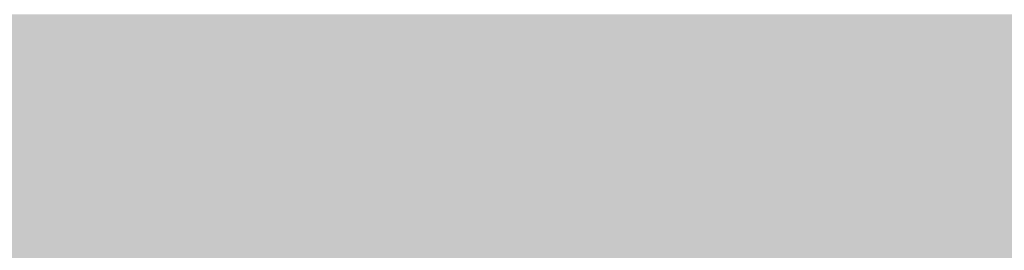
# Model space of a CAD drawing. Units: feet. Extents: x 3168 to 4724, y 827 to 1477.
# Tile 41 of 256: x 3270.273 to 3273.072, y 1098.344 to 1099.001. Entities that reach past the tile are written whole.
import ezdxf

# ---------------------------------------------------------------- set-up
doc = ezdxf.new("R2010")
doc.units = ezdxf.units.FT
doc.layers.add('A-ELEV', color=7, linetype='Continuous', lineweight=35)
doc.layers.add('A-ELEV-PATT', color=8, linetype='Continuous', lineweight=13)

msp = doc.modelspace()

# ---------------------------------------------------------------- hatches: boundary and pattern name
at = {"layer": 'A-ELEV-PATT'}
h = msp.add_hatch(color=256, dxfattribs=at)
h.dxf.hatch_style = 1
edge = h.paths.add_edge_path()
edge.add_ellipse((3552.9058, 979.2201), major_axis=(36.7449, 0), ratio=0.4848485, start_angle=0, end_angle=360)
edge = h.paths.add_edge_path()
edge.add_ellipse((3559.8916, 929.2523), major_axis=(36.7449, 0), ratio=0.4848485, start_angle=0, end_angle=360)
edge = h.paths.add_edge_path()
edge.add_line((3299.3168, 1198.6061), (3479.9167, 1198.6061))
edge.add_line((3479.9167, 1198.6061), (3479.9167, 1209.8686))
edge.add_spline(control_points=[(3479.9167, 1209.8686), (3464.3012, 1209.8686), (3448.6856, 1209.8686), (3410.9491, 1209.8686), (3388.8282, 1209.8686), (3355.6469, 1209.8686), (3344.5864, 1209.8686), (3327.9957, 1209.8686), (3322.4655, 1209.8686), (3314.1702, 1209.8686), (3311.4051, 1209.8686), (3307.2574, 1209.8686), (3305.8748, 1209.8686), (3303.801, 1209.8686), (3303.1097, 1209.8686), (3302.0728, 1209.8686), (3301.7272, 1209.8686), (3301.2087, 1209.8686), (3301.0359, 1209.8686), (3300.7767, 1209.8686), (3300.6903, 1209.8686), (3300.5606, 1209.8686), (3300.5174, 1209.8686), (3300.4526, 1209.8686), (3300.431, 1209.8686), (3300.3986, 1209.8686), (3300.3878, 1209.8686), (3300.3662, 1209.8686), (3300.3457, 1209.8686), (3300.3455, 1209.8686), (3300.3455, 1209.8686), (3300.3433, 1209.8686), (3300.3411, 1209.8686), (3300.3379, 1209.8686), (3300.3368, 1209.8686), (3300.3339, 1209.8686), (3300.3321, 1209.8686), (3300.3255, 1209.8686), (3300.3207, 1209.8686), (3300.3109, 1209.8686), (3300.306, 1209.8686), (3300.2905, 1209.8686), (3300.28, 1209.8686), (3300.2324, 1209.8688), (3300.1953, 1209.869), (3299.9511, 1209.8706), (3299.7448, 1209.8743), (3299.4368, 1209.8833), (3299.3344, 1209.8868), (3299.1811, 1209.8929), (3299.13, 1209.8951), (3298.6522, 1209.9168), (3298.2295, 1209.9457), (3297.6016, 1210.0024), (3297.3934, 1210.0235), (3297.0827, 1210.0583), (3296.9793, 1210.0705), (3296.293, 1210.1549), (3295.7181, 1210.2434), (3294.8687, 1210.3989), (3294.5877, 1210.4545), (3294.1693, 1210.5433), (3294.0304, 1210.5739), (3291.7071, 1211.1012), (3289.6536, 1211.8134), (3285.7763, 1213.564), (3283.9514, 1214.6035), (3280.5122, 1216.9801), (3278.8972, 1218.3176), (3276.3799, 1220.8295), (3275.416, 1221.9177), (3274.0393, 1223.7077), (3273.581, 1224.3495), (3273.1432, 1225.0163)], knot_values=[39.119033, 39.119033, 39.119033, 39.119033, 39.286353, 39.286353, 39.523379, 39.523379, 39.641892, 39.641892, 39.701148, 39.701148, 39.730777, 39.730777, 39.745591, 39.745591, 39.752998, 39.752998, 39.756701, 39.756701, 39.758553, 39.758553, 39.759479, 39.759479, 39.759942, 39.759942, 39.760173, 39.760173, 39.760289, 39.760289, 39.760405, 39.760405, 39.760463, 39.760463, 39.763389, 39.763389, 39.764851, 39.764851, 39.767304, 39.767304, 39.773825, 39.773825, 39.78057, 39.78057, 39.79477, 39.79477, 39.845194, 39.845194, 40.126715, 40.126715, 40.267476, 40.267476, 40.337856, 40.337856, 40.927023, 40.927023, 41.221606, 41.221606, 41.368898, 41.368898, 42.202622, 42.202622, 42.619485, 42.619485, 42.827916, 42.827916, 46.118323, 46.118323, 49.408731, 49.408731, 52.699139, 52.699139, 54.927489, 54.927489, 56.104228, 56.104228, 56.104228, 56.104228], weights=[1, 1, 1, 1, 1, 1, 1, 1, 1, 1, 1, 1, 1, 1, 1, 1, 1, 1, 1, 1, 1, 1, 1, 1, 1, 1, 1, 1, 1, 1, 1, 1, 1, 1, 1, 1, 1, 1, 1, 1, 1, 1, 1, 1, 1, 1, 1, 1, 1, 1, 1, 1, 1, 1, 1, 1, 1, 1, 1, 1, 1, 1, 1, 1, 1, 1, 1, 1, 1, 1, 1, 1, 1, 1], degree=3, periodic=0)
edge.add_line((3273.1432, 1225.0163), (3273.1432, 1099.0163))
edge.add_line((3273.1432, 1099.0163), (3299.3168, 1099.0163))
edge.add_line((3299.3168, 1099.0163), (3299.3168, 1198.6061))
edge = h.paths.add_edge_path()
edge.add_line((3304.7584, 1324.1581), (3479.9167, 1324.1581))
edge.add_line((3479.9167, 1324.1581), (3479.9167, 1335.7146))
edge.add_line((3479.9167, 1335.7146), (3269.1616, 1335.7146))
edge.add_spline(control_points=[(3269.1616, 1335.7146), (3264.0242, 1335.7146), (3258.3641, 1328.9582), (3259.2643, 1323.9003)], knot_values=[0, 0, 0, 0, 15.412191, 15.412191, 15.412191, 15.412191], degree=3, periodic=0)
edge.add_line((3259.2643, 1323.9003), (3265.5168, 1288.7691))
edge.add_line((3265.5168, 1288.7691), (3275.2651, 1261.5456))
edge.add_line((3275.2651, 1261.5456), (3304.7584, 1261.5456))
edge.add_line((3304.7584, 1261.5456), (3304.7584, 1324.1581))
h = msp.add_hatch(color=256, dxfattribs=at)
h.dxf.hatch_style = 1
h.paths.add_polyline_path([(3384.5252, 1099.0163), (3335.0292, 1099.0163), (3299.3168, 1099.0163), (3273.1432, 1099.0163), (3217.5654, 1099.0163), (3168.0693, 827.1163), (3335.0292, 827.1163)])

# ---------------------------------------------------------------- linework, layer by layer
at = {"layer": 'A-ELEV'}
msp.add_open_spline([(3808.5202, 1099.0163), (3808.5202, 1141.4132), (3808.5202, 1183.8102), (3808.5202, 1226.6353), (3808.5202, 1227.0636), (3808.5202, 1227.4918), (3811.4919, 1248.9947), (3814.4635, 1270.4975), (3817.4652, 1292.2176), (3817.4952, 1292.4348), (3817.5253, 1292.652), (3817.5728, 1310.1067), (3817.6203, 1327.5615), (3817.6679, 1345.0163), (3817.6679, 1345.458), (3817.6679, 1345.8996), (3817.6679, 1346.456), (3817.6679, 1346.5708), (3817.6679, 1346.7529), (3817.6679, 1346.8201), (3817.6679, 1346.9349), (3817.6679, 1346.9823), (3817.6679, 1347.0386), (3817.6679, 1347.0474), (3817.6679, 1347.0737), (3817.6679, 1347.0593), (3817.6679, 1347.0615), (3817.6679, 1347.0627), (3817.6679, 1347.066), (3817.6679, 1347.0683), (3817.6679, 1347.075), (3817.6679, 1347.0795), (3817.6678, 1347.0929), (3817.6678, 1347.1019), (3817.6678, 1347.1288), (3817.6677, 1347.1467), (3817.6674, 1347.2004), (3817.6672, 1347.2362), (3817.6661, 1347.3434), (3817.665, 1347.4147), (3817.6608, 1347.6281), (3817.6566, 1347.7697), (3817.64, 1348.1925), (3817.6235, 1348.4716), (3817.5591, 1349.3001), (3817.4961, 1349.8406), (3817.2554, 1351.4242), (3817.0263, 1352.4288), (3816.3069, 1354.8889), (3815.7437, 1356.2687), (3814.464, 1358.8192), (3813.7464, 1359.991), (3812.1958, 1362.1723), (3811.3622, 1363.1821), (3809.5888, 1365.069), (3808.6488, 1365.9461), (3806.6543, 1367.5796), (3805.5997, 1368.3362), (3803.3529, 1369.7223), (3802.1605, 1370.3524), (3799.6008, 1371.4536), (3798.2327, 1371.9255), (3795.2801, 1372.6346), (3793.6931, 1372.8721), (3791.8694, 1372.9265), (3791.7409, 1372.9292), (3791.3534, 1372.9341), (3791.0927, 1372.9329), (3790.3041, 1372.9151), (3789.7695, 1372.8842), (3789.2092, 1372.8302), (3789.1906, 1372.8284), (3789.1349, 1372.8229), (3789.0977, 1372.8191), (3789.0484, 1372.814), (3789.0364, 1372.8127), (3789.0003, 1372.8089), (3788.9761, 1372.8063), (3788.9494, 1372.8034), (3788.9468, 1372.8031), (3788.9426, 1372.8027), (3788.941, 1372.8025), (3788.9386, 1372.8022), (3788.9378, 1372.8021), (3788.9354, 1372.8019), (3788.8675, 1372.7944), (3788.7569, 1372.7822), (3788.7015, 1372.7761), (3788.5355, 1372.7579), (3788.4249, 1372.7457), (3788.0929, 1372.7092), (3787.8715, 1372.6848), (3787.2075, 1372.6118), (3786.7648, 1372.5631), (3785.4368, 1372.417), (3784.5515, 1372.3196), (3781.8954, 1372.0274), (3780.1247, 1371.8327), (3774.8126, 1371.2483), (3771.2713, 1370.8587), (3760.6471, 1369.69), (3753.5643, 1368.9109), (3732.316, 1366.5735), (3718.1504, 1365.0152), (3694.0068, 1362.3593), (3684.0287, 1361.2617), (3674.0506, 1360.1641), (3664.6007, 1360.1641), (3655.1508, 1360.1641), (3626.8011, 1360.1641), (3607.9013, 1360.1641), (3551.2019, 1360.1641), (3513.4023, 1360.1641), (3467.7252, 1360.1641), (3459.8476, 1360.1641), (3436.2149, 1360.1641), (3420.4597, 1360.1641), (3373.1943, 1360.1641), (3341.6839, 1360.1641), (3302.8482, 1360.1641), (3295.5227, 1360.1641), (3286.0383, 1360.1641), (3283.8794, 1360.1641), (3277.4026, 1360.1641), (3273.0848, 1360.1641), (3267.7329, 1360.1641), (3266.6988, 1360.1641), (3263.5965, 1360.1641), (3261.5284, 1360.1641), (3259.2369, 1360.1641), (3259.0137, 1360.1641), (3258.344, 1360.1641), (3257.8975, 1360.1641), (3257.431, 1360.1641), (3257.411, 1360.1641), (3257.3706, 1360.1641), (3257.3755, 1360.1641), (3257.3746, 1360.1641), (3257.3739, 1360.1641), (3257.372, 1360.1641), (3257.3706, 1360.1641), (3257.3667, 1360.1641), (3257.364, 1360.1641), (3257.3561, 1360.1641), (3257.3508, 1360.164), (3257.335, 1360.164), (3257.3244, 1360.164), (3257.2928, 1360.1639), (3257.2717, 1360.1638), (3257.2084, 1360.1634), (3257.1663, 1360.163), (3257.0402, 1360.1614), (3256.9563, 1360.1598), (3256.7055, 1360.1534), (3256.5392, 1360.147), (3256.0436, 1360.1219), (3255.7173, 1360.0971), (3254.7524, 1360.0005), (3254.128, 1359.9065), (3252.1801, 1359.5253), (3250.9416, 1359.144), (3248.6702, 1358.2433), (3247.6357, 1357.7238), (3245.7326, 1356.6035), (3244.8634, 1356.0021), (3243.2531, 1354.7429), (3242.512, 1354.0847), (3240.7511, 1352.3448), (3239.801, 1351.2296), (3238.0878, 1348.8724), (3237.3247, 1347.6304), (3235.9825, 1344.9716), (3235.4022, 1343.5549), (3234.5911, 1340.8155), (3234.3109, 1339.5435), (3233.9765, 1336.8026), (3233.9221, 1335.3309), (3234.1489, 1332.5913), (3234.3495, 1331.3672), (3234.7199, 1329.9994), (3234.7524, 1329.8834), (3234.8536, 1329.5348), (3234.9259, 1329.3017), (3235.0248, 1329.0026), (3235.0469, 1328.9369), (3235.0776, 1328.8472), (3235.0859, 1328.8232), (3235.1109, 1328.7511), (3235.1278, 1328.703), (3235.148, 1328.6462), (3235.1511, 1328.6376), (3235.1561, 1328.6235), (3235.1581, 1328.618), (3235.1602, 1328.612), (3235.1656, 1328.5969), (3235.1801, 1328.5565), (3235.1903, 1328.5281), (3235.2208, 1328.4429), (3235.2411, 1328.3862), (3235.3021, 1328.2159), (3235.3427, 1328.1023), (3235.4647, 1327.7617), (3235.546, 1327.5346), (3235.79, 1326.8534), (3235.9526, 1326.3992), (3236.4405, 1325.0367), (3236.7657, 1324.1284), (3237.7415, 1321.4034), (3238.392, 1319.5868), (3240.3435, 1314.1369), (3241.6445, 1310.5036), (3245.5476, 1299.6037), (3248.1496, 1292.3371), (3255.9557, 1270.5374), (3261.1598, 1256.0042), (3267.3876, 1238.612), (3268.4114, 1235.7529), (3269.5104, 1232.6839), (3269.5856, 1232.4739), (3269.7066, 1232.1359), (3269.7524, 1232.0079), (3269.8273, 1231.7987), (3269.8564, 1231.7176), (3269.9063, 1231.5781), (3269.9272, 1231.5198), (3269.9725, 1231.3934), (3269.9968, 1231.3254), (3270.0265, 1231.2425), (3270.0318, 1231.2277), (3270.0403, 1231.204), (3270.0392, 1231.207), (3270.0394, 1231.2066), (3270.0394, 1231.2064), (3270.0396, 1231.2058), (3270.0398, 1231.2055), (3270.0402, 1231.2043), (3270.0404, 1231.2036), (3270.0413, 1231.2013), (3270.0418, 1231.1998), (3270.0434, 1231.1953), (3270.0445, 1231.1922), (3270.0478, 1231.1832), (3270.0499, 1231.1771), (3270.0564, 1231.159), (3270.0608, 1231.147), (3270.0739, 1231.1108), (3270.0826, 1231.0867), (3270.1089, 1231.0144), (3270.1266, 1230.9663), (3270.1799, 1230.8225), (3270.2159, 1230.7269), (3270.3253, 1230.4415), (3270.4, 1230.2528), (3270.6292, 1229.6914), (3270.7889, 1229.3235), (3271.2865, 1228.2383), (3271.6431, 1227.5398), (3272.7759, 1225.5153), (3273.6142, 1224.2605), (3275.416, 1221.9177), (3276.3799, 1220.8295), (3278.8972, 1218.3176), (3280.5122, 1216.9801), (3283.9514, 1214.6035), (3285.7763, 1213.564), (3289.6536, 1211.8134), (3291.7071, 1211.1012), (3294.0304, 1210.5739), (3294.1693, 1210.5433), (3294.5877, 1210.4545), (3294.8687, 1210.3989), (3295.7181, 1210.2434), (3296.293, 1210.1549), (3296.9793, 1210.0705), (3297.0827, 1210.0583), (3297.3934, 1210.0235), (3297.6016, 1210.0024), (3298.2295, 1209.9457), (3298.6522, 1209.9168), (3299.13, 1209.8951), (3299.1811, 1209.8929), (3299.3344, 1209.8868), (3299.4368, 1209.8833), (3299.7448, 1209.8743), (3299.9511, 1209.8706), (3300.1953, 1209.869), (3300.2324, 1209.8688), (3300.28, 1209.8686), (3300.2905, 1209.8686), (3300.306, 1209.8686), (3300.3109, 1209.8686), (3300.3207, 1209.8686), (3300.3255, 1209.8686), (3300.3321, 1209.8686), (3300.3339, 1209.8686), (3300.3368, 1209.8686), (3300.3379, 1209.8686), (3300.3411, 1209.8686), (3300.3433, 1209.8686), (3300.3455, 1209.8686), (3300.3455, 1209.8686), (3300.3457, 1209.8686), (3300.3662, 1209.8686), (3300.3878, 1209.8686), (3300.3986, 1209.8686), (3300.431, 1209.8686), (3300.4526, 1209.8686), (3300.5174, 1209.8686), (3300.5606, 1209.8686), (3300.6903, 1209.8686), (3300.7767, 1209.8686), (3301.0359, 1209.8686), (3301.2087, 1209.8686), (3301.7272, 1209.8686), (3302.0728, 1209.8686), (3303.1097, 1209.8686), (3303.801, 1209.8686), (3305.8748, 1209.8686), (3307.2574, 1209.8686), (3311.4051, 1209.8686), (3314.1702, 1209.8686), (3322.4655, 1209.8686), (3327.9957, 1209.8686), (3344.5864, 1209.8686), (3355.6469, 1209.8686), (3388.8282, 1209.8686), (3410.9491, 1209.8686), (3477.3119, 1209.8686), (3521.5537, 1209.8686), (3566.8362, 1209.8686), (3567.8769, 1209.8686), (3570.999, 1209.8686), (3573.0804, 1209.8686), (3575.7814, 1209.8686), (3576.4009, 1209.8686), (3577.2958, 1209.8686), (3577.5712, 1209.8686), (3578.3971, 1209.8686), (3578.9478, 1209.8686), (3579.7565, 1209.8686), (3580.0145, 1209.8686), (3580.3427, 1209.8686), (3580.3269, 1209.8686), (3580.3272, 1209.8686), (3580.3273, 1209.8686), (3580.3278, 1209.8686), (3580.3281, 1209.8686), (3580.329, 1209.8686), (3580.3296, 1209.8686), (3580.3314, 1209.8686), (3580.3327, 1209.8686), (3580.3363, 1209.8686), (3580.3388, 1209.8686), (3580.3461, 1209.8686), (3580.351, 1209.8686), (3580.3657, 1209.8685), (3580.3754, 1209.8685), (3580.4048, 1209.8684), (3580.4244, 1209.8684), (3580.4832, 1209.8681), (3580.5224, 1209.8678), (3580.6404, 1209.8666), (3580.7192, 1209.8655), (3580.9563, 1209.8608), (3581.1152, 1209.8561), (3581.5942, 1209.8372), (3581.9164, 1209.8183), (3582.8899, 1209.7424), (3583.548, 1209.6662), (3585.5318, 1209.3606), (3586.8672, 1209.0539), (3589.4715, 1208.2525), (3590.7402, 1207.7579), (3591.9955, 1207.1588), (3592.0578, 1207.1287), (3592.2442, 1207.038), (3592.3677, 1206.9766), (3592.7353, 1206.7904), (3592.9768, 1206.6631), (3593.2445, 1206.5164), (3593.2747, 1206.4998), (3593.3651, 1206.4498), (3593.4251, 1206.4163), (3593.6043, 1206.3153), (3593.7227, 1206.2472), (3593.8572, 1206.1684), (3593.8744, 1206.1583), (3593.9257, 1206.128), (3593.9599, 1206.1078), (3594.0621, 1206.0469), (3594.1298, 1206.0061), (3594.2084, 1205.9582), (3594.2197, 1205.9513), (3594.2534, 1205.9307), (3594.2758, 1205.9169), (3594.343, 1205.8755), (3594.3876, 1205.8479), (3594.4336, 1205.819), (3594.4353, 1205.818), (3594.4402, 1205.8149), (3594.4435, 1205.8129), (3594.4471, 1205.8106), (3594.4475, 1205.8103), (3594.4487, 1205.8096), (3594.4495, 1205.8091), (3594.4504, 1205.8086), (3594.4505, 1205.8085), (3594.4506, 1205.8084), (3594.4674, 1205.7979), (3594.4933, 1205.7817), (3594.5062, 1205.7736), (3594.545, 1205.7492), (3594.5709, 1205.733), (3594.6485, 1205.6844), (3594.7002, 1205.652), (3594.8554, 1205.5547), (3594.9589, 1205.4898), (3595.2694, 1205.2953), (3595.4763, 1205.1656), (3596.0972, 1204.7765), (3596.5111, 1204.5171), (3597.7528, 1203.7388), (3598.5807, 1203.22), (3601.0642, 1201.6636), (3602.7198, 1200.6259), (3607.6868, 1197.513), (3610.9981, 1195.4377), (3620.932, 1189.2119), (3627.5546, 1185.0614), (3647.4225, 1172.6097), (3660.6678, 1164.3086), (3700.4035, 1139.4053), (3726.894, 1122.8031), (3757.2057, 1103.8061), (3761.027, 1101.4112), (3764.8482, 1099.0163), (3745.3283, 1099.0163), (3725.8083, 1099.0163), (3706.2884, 1099.0163), (3706.2884, 1108.4532), (3706.2884, 1117.8902), (3706.2884, 1127.3271), (3710.7508, 1127.3271), (3715.2131, 1127.3271), (3719.6755, 1127.3271)], degree=3, knots=[0, 0, 0, 0, 0.982037, 0.982037, 0.991957, 0.991957, 0.991957, 1.966522, 1.966522, 1.976367, 1.976367, 1.976367, 2.976367, 2.976367, 2.976367, 3.00169, 3.00169, 3.008272, 3.008272, 3.012129, 3.012129, 3.014851, 3.014851, 3.015353, 3.015353, 3.016359, 3.016359, 3.017365, 3.017365, 3.019376, 3.019376, 3.023398, 3.023398, 3.031442, 3.031442, 3.047531, 3.047531, 3.079708, 3.079708, 3.144063, 3.144063, 3.272772, 3.272772, 3.53019, 3.53019, 4.045026, 4.045026, 5.074698, 5.074698, 6.700878, 6.700878, 8.327058, 8.327058, 9.953238, 9.953238, 11.579418, 11.579418, 13.205598, 13.205598, 14.831778, 14.831778, 16.457958, 16.457958, 18.084138, 18.084138, 18.206872, 18.206872, 18.45234, 18.45234, 18.943275, 18.943275, 18.960093, 18.960093, 18.993729, 18.993729, 19.00461, 19.00461, 19.026374, 19.026374, 19.028737, 19.028737, 19.03018, 19.03018, 19.030897, 19.030897, 19.032332, 19.032332, 19.033766, 19.033766, 19.036636, 19.036636, 19.042374, 19.042374, 19.053851, 19.053851, 19.076805, 19.076805, 19.122714, 19.122714, 19.21453, 19.21453, 19.398163, 19.398163, 19.765429, 19.765429, 20.024128, 20.024128, 20.024128, 20.092031, 20.092031, 20.227836, 20.227836, 20.499446, 20.499446, 20.556051, 20.556051, 20.66926, 20.66926, 20.895678, 20.895678, 20.948316, 20.948316, 20.963829, 20.963829, 20.994855, 20.994855, 21.002285, 21.002285, 21.017146, 21.017146, 21.01875, 21.01875, 21.021959, 21.021959, 21.022102, 21.022102, 21.022249, 21.022249, 21.022708, 21.022708, 21.023627, 21.023627, 21.025464, 21.025464, 21.029138, 21.029138, 21.036486, 21.036486, 21.051183, 21.051183, 21.080575, 21.080575, 21.139361, 21.139361, 21.256932, 21.256932, 21.492073, 21.492073, 21.962356, 21.962356, 23.01002, 23.01002, 24.057684, 24.057684, 25.105348, 25.105348, 26.153011, 26.153011, 27.776787, 27.776787, 29.400562, 29.400562, 31.024337, 31.024337, 32.278801, 32.278801, 33.533265, 33.533265, 34.467568, 34.467568, 34.553971, 34.553971, 34.726776, 34.726776, 34.775309, 34.775309, 34.793079, 34.793079, 34.82862, 34.82862, 34.834979, 34.834979, 34.839039, 34.839039, 34.839411, 34.839411, 34.840285, 34.840285, 34.842034, 34.842034, 34.845531, 34.845531, 34.852525, 34.852525, 34.866512, 34.866512, 34.894488, 34.894488, 34.950439, 34.950439, 35.062342, 35.062342, 35.286147, 35.286147, 35.733758, 35.733758, 35.821815, 35.821815, 35.828283, 35.828283, 35.832225, 35.832225, 35.834724, 35.834724, 35.836521, 35.836521, 35.838617, 35.838617, 35.839073, 35.839073, 35.839345, 35.839345, 35.839617, 35.839617, 35.840161, 35.840161, 35.841249, 35.841249, 35.843425, 35.843425, 35.847778, 35.847778, 35.856482, 35.856482, 35.873891, 35.873891, 35.908709, 35.908709, 35.978345, 35.978345, 36.117617, 36.117617, 36.396161, 36.396161, 36.953248, 36.953248, 38.067423, 38.067423, 40.295772, 40.295772, 42.524122, 42.524122, 45.81453, 45.81453, 49.104937, 49.104937, 52.395345, 52.395345, 52.603776, 52.603776, 53.020639, 53.020639, 53.854363, 53.854363, 54.001655, 54.001655, 54.296238, 54.296238, 54.885405, 54.885405, 54.955785, 54.955785, 55.096546, 55.096546, 55.378067, 55.378067, 55.42849, 55.42849, 55.442691, 55.442691, 55.449436, 55.449436, 55.455957, 55.455957, 55.458409, 55.458409, 55.459872, 55.459872, 55.462798, 55.462798, 55.462856, 55.462856, 55.462972, 55.462972, 55.463088, 55.463088, 55.463319, 55.463319, 55.463782, 55.463782, 55.464708, 55.464708, 55.46656, 55.46656, 55.470263, 55.470263, 55.47767, 55.47767, 55.492484, 55.492484, 55.522112, 55.522112, 55.581369, 55.581369, 55.699882, 55.699882, 55.936907, 55.936907, 56.410959, 56.410959, 56.42211, 56.42211, 56.444413, 56.444413, 56.451051, 56.451051, 56.454001, 56.454001, 56.459901, 56.459901, 56.462666, 56.462666, 56.463418, 56.463418, 56.464171, 56.464171, 56.465675, 56.465675, 56.468684, 56.468684, 56.474702, 56.474702, 56.486738, 56.486738, 56.51081, 56.51081, 56.558955, 56.558955, 56.655243, 56.655243, 56.847821, 56.847821, 57.232975, 57.232975, 58.003284, 58.003284, 59.543901, 59.543901, 62.625137, 62.625137, 68.787607, 68.787607, 74.950078, 74.950078, 75.27336, 75.27336, 75.919923, 75.919923, 77.213051, 77.213051, 77.377769, 77.377769, 77.707206, 77.707206, 78.366079, 78.366079, 78.462532, 78.462532, 78.655436, 78.655436, 79.041245, 79.041245, 79.105735, 79.105735, 79.234714, 79.234714, 79.492672, 79.492672, 79.502197, 79.502197, 79.521249, 79.521249, 79.523534, 79.523534, 79.528103, 79.528103, 79.528682, 79.528682, 79.528885, 79.528885, 79.529089, 79.529089, 79.529495, 79.529495, 79.530308, 79.530308, 79.531935, 79.531935, 79.535187, 79.535187, 79.541693, 79.541693, 79.554704, 79.554704, 79.580725, 79.580725, 79.632769, 79.632769, 79.736856, 79.736856, 79.94503, 79.94503, 80.361377, 80.361377, 80.421435, 80.421435, 80.421435, 81.421435, 81.421435, 81.421435, 82.421435, 82.421435, 82.421435, 83.421435, 83.421435, 83.421435, 83.421435], dxfattribs=at)

doc.saveas('drawing.dxf')
